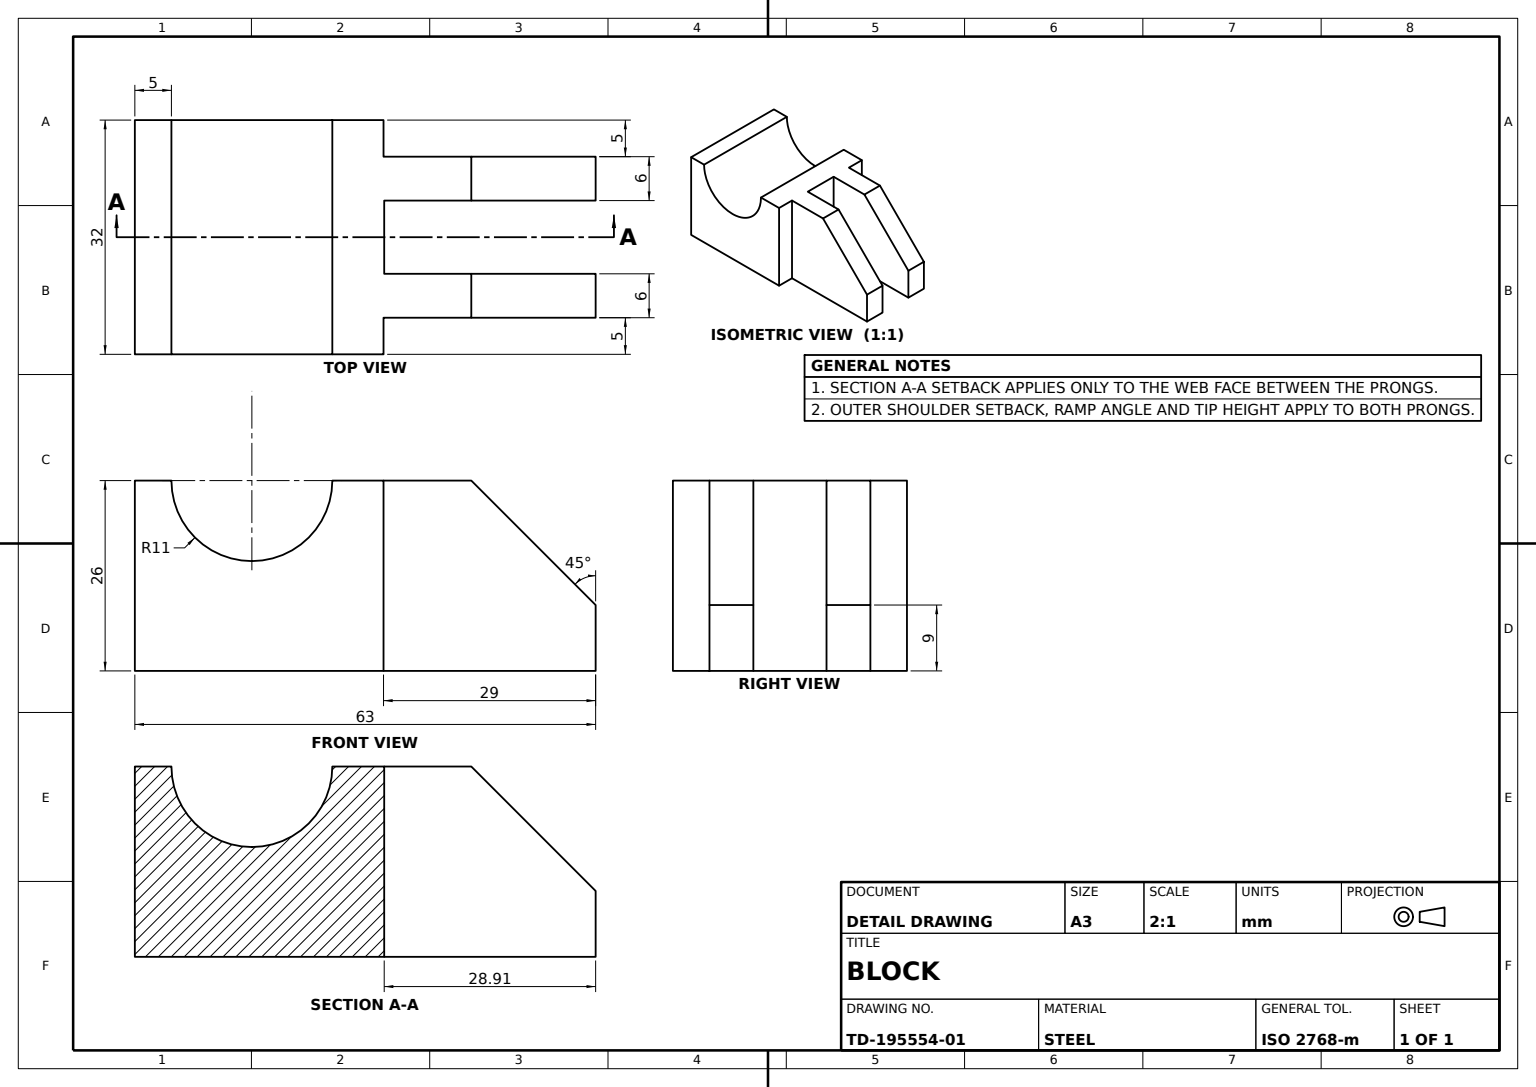
SolidWorks part; units mm, degrees
material "Plain Carbon Steel"
ref_plane "Front Plane" through (0, 0, 0) normal (0, 0, 1) x (1, 0, 0)
ref_plane "Top Plane" through (0, 0, 0) normal (0, 1, 0) x (1, 0, 0)
ref_plane "Right Plane" through (0, 0, 0) normal (1, 0, 0) x (0, 0, -1)
sketch "Base Block Profile 63x32" plane through (0, 0, 0) normal (0, 0, 1) x (1, 0, 0)
  line L1 (-31.5, 16) -> (31.5, 16)
  line L2 (-31.5, 16) -> (-31.5, -16)
  line L3 (-31.5, -16) -> (31.5, -16)
  line L4 (31.5, 16) -> (31.5, -16)
  line L5 (-31.5, 16) -> (31.5, -16) construction
  line L6 (-31.5, -16) -> (31.5, 16) construction
  point P0 (0, 0)
  dimension "D1" = 32
  dimension "D2" = 63
extrude "Base Block 63x32x26" add sketch "Base Block Profile 63x32" along normal blind 26
sketch "Bore Slot Profile" plane through (0, -16, 0) normal (0, -1, 0) x (1, 0, 0)
  line L0 (-31.5, 0) -> (-31.5, 7.3393)
  line L1 (-31.5, 26) -> (-31.5, 0) construction
  line L2 (31.5, 0) -> (31.5, 26)
  line L3 (31.5, 26) -> (26.5, 26)
  line L4 (-31.5, 26) -> (31.5, 26) construction
  line L5 (26.5, 26) -> (4.5, 26)
  line L6 (31.5, 26) -> (-2.5, 26)
  line L8 (-31.5, 0) -> (31.5, 0) construction
  arc A0 (4.5, 26) -> (26.5, 26) centre (15.5, 26) ccw
  line M5 (31.5, 26) -> (-31.5, 26)
  dimension "D3" = 34
  dimension "D1" = 5
  dimension "D2" = 22
  dimension "D4" = 7.3393
extrude "Bore Slot Cut" cut sketch "Bore Slot Profile" against normal blind 32 contours A0 M5
sketch "Rectangular Slot Profile 17x9" plane through (0, -16, 0) normal (0, -1, 0) x (-1, 0, 0)
  line L1 (31.5, -26) -> (-4.5, -26) construction
  line L2 (14.5, -26) -> (31.5, -26)
  line L4 (31.5, 0) -> (31.5, -9)
  line L5 (31.5, -26) -> (31.5, 0) construction
  line L6 (31.5, -9) -> (14.5, -26)
  line L7 (31.5, -9) -> (31.5, -26)
  line M6 (-4.5, -26) -> (31.5, -26)
  line M7 (31.5, -26) -> (31.5, 0)
  dimension "D1" = 17
  dimension "D2" = 9
extrude "Rectangular Slot 17x9" cut sketch "Rectangular Slot Profile 17x9" against normal blind 32 contours L6 M7 M6
sketch "Side Step Profile" plane through (0, 0, 0) normal (0, 0, -1) x (-1, 0, 0)
  line L1 (31.5, 16) -> (2.5, 16)
  line L2 (31.5, 16) -> (31.5, 11)
  line L3 (31.5, 11) -> (2.5, 11)
  line L4 (2.5, 16) -> (2.5, 11)
  line L5 (31.5, -16) -> (2.5, -16)
  line L6 (31.5, -16) -> (31.5, -11)
  line L7 (31.5, -11) -> (2.5, -11)
  line L8 (2.5, -16) -> (2.5, -11)
  dimension "D1" = 5
  dimension "D2" = 29
  dimension "D3" = 5
extrude "Side Step Cut" cut sketch "Side Step Profile" against normal through all
sketch "Side Groove Profile" plane through (0, 0, 0) normal (0, 0, -1) x (-1, 0, 0)
  line L0 (31.5, 0) -> (31.5, 5)
  line L1 (31.5, 11) -> (31.5, -11) construction
  line L2 (31.5, 0) -> (31.5, -5.0029)
  line L4 (31.5, 11) -> (2.5924, 11)
  line L5 (31.5, 11) -> (31.5, 5)
  line L6 (31.5, 5) -> (2.5924, 5)
  line L7 (2.5924, 11) -> (2.5924, 5)
  line L8 (31.5, -11) -> (2.5924, -11)
  line L9 (31.5, -11) -> (31.5, -5.0029)
  line L10 (31.5, -5.0029) -> (2.5924, -5.0029)
  line L11 (2.5924, -11) -> (2.5924, -5.0029)
  line L12 (2.5924, 5) -> (31.5, 5)
  line L13 (2.5924, 5) -> (2.5924, -5.0029)
  line L14 (2.5924, -5.0029) -> (31.5, -5.0029)
  line L15 (31.5, 5) -> (31.5, -5.0029)
  line M5 (31.5, -11) -> (31.5, 11)
  dimension "D1" = 5.0029
  dimension "D2" = 5
  dimension "D3" = 28.9076
extrude "Side Groove Cut" cut sketch "Side Groove Profile" against normal through all contours L6 L13 L10 M5
